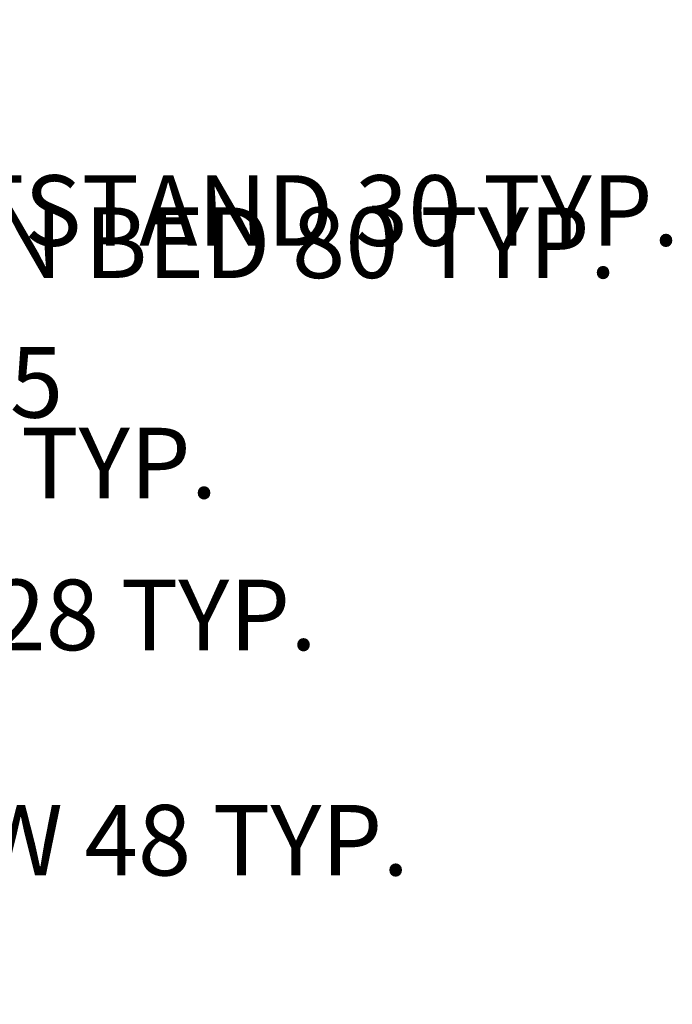
# Model space of a CAD drawing. Units: inches. Extents: x 1173 to 2157, y 515 to 1129.
# Tile 13 of 13: x 1824 to 2157, y 578 to 1080. Entities that reach past the tile are written whole.
import ezdxf

# ---------------------------------------------------------------- set-up
doc = ezdxf.new("R2010")
doc.units = ezdxf.units.IN
doc.header["$MEASUREMENT"] = 0
doc.layers.add('A-ANNO-DIMS', color=2, linetype='Continuous', lineweight=18)
doc.styles.get("Standard").update_dxf_attribs({"font": 'arial.ttf'})
doc.dimstyles.get("Standard").update_dxf_attribs({"dimtxt": 36, "dimasz": 0.18, "dimexe": 0.18, "dimexo": 0.0625, "dimgap": 0.09, "dimtad": 0, "dimtih": 1, "dimtoh": 1, "dimdec": 0, "dimrnd": 72, "dimzin": 0, "dimdsep": 46, "dimlunit": 3, "dimtxsty": 'Standard', "dimcen": 2, "dimadec": 0, "dimazin": 0, "dimtfac": 1, "dimtdec": 0, "dimtofl": 0, "dimtmove": 0, "dimatfit": 3, "dimfxl": 1, "dimtolj": 1, "dimtzin": 0, "dimarcsym": 0})

# ---------------------------------------------------------------- blocks, each defined once
blk = doc.blocks.new('*D26')
at = {"layer": 'A-ANNO-DIMS', "color": 0, "lineweight": -2, "transparency": 16777216}
for p, q in [((1577.15, 654.34), (1577.15, 661.66)), ((1577.33, 661.48), (1624.97, 661.48)), ((1625.15, 654.34), (1625.15, 661.66)), ((1625.15, 661.48), (1625.33, 661.48))]:
    blk.add_line(p, q, dxfattribs=at)
at = {"layer": 'A-ANNO-DIMS', "color": 0, "transparency": 16777216}
for points in [[(1577.33, 661.51), (1577.33, 661.45), (1577.15, 661.48)], [(1624.97, 661.51), (1624.97, 661.45), (1625.15, 661.48)]]:
    blk.add_solid(points, dxfattribs=at)
at = {"layer": 'Defpoints', "color": 0, "transparency": 16777216}
for p in [(1625.15, 661.48), (1577.15, 654.28), (1625.15, 654.28)]:
    blk.add_point(p, dxfattribs=at)
at = {"layer": 'A-ANNO-DIMS', "color": 0, "transparency": 16777216, "insert": (1831.09, 661.48), "char_height": 36, "attachment_point": 5}
blk.add_mtext('\\A1;WINDOW 48 TYP.', dxfattribs=at)
blk = doc.blocks.new('*D28')
at = {"layer": 'A-ANNO-DIMS', "color": 0, "lineweight": -2, "transparency": 16777216}
for p, q in [((1581.66, 978.31), (1581.66, 966.19)), ((1661.66, 978.31), (1661.66, 966.19)), ((1581.84, 966.37), (1661.48, 966.37)), ((1661.66, 966.37), (1661.84, 966.37))]:
    blk.add_line(p, q, dxfattribs=at)
at = {"layer": 'A-ANNO-DIMS', "color": 0, "transparency": 16777216}
for points in [[(1581.84, 966.4), (1581.84, 966.34), (1581.66, 966.37)], [(1661.48, 966.4), (1661.48, 966.34), (1661.66, 966.37)]]:
    blk.add_solid(points, dxfattribs=at)
at = {"layer": 'Defpoints', "color": 0, "transparency": 16777216}
for p in [(1581.66, 978.37), (1661.66, 978.37), (1661.66, 966.37)]:
    blk.add_point(p, dxfattribs=at)
at = {"layer": 'A-ANNO-DIMS', "color": 0, "transparency": 16777216, "insert": (1904.61, 966.37), "char_height": 36, "attachment_point": 5}
blk.add_mtext('\\A1;QUEEN BED 80 TYP.', dxfattribs=at)
blk = doc.blocks.new('*D32')
at = {"layer": 'A-ANNO-DIMS', "color": 0, "lineweight": -2, "transparency": 16777216}
for p, q in [((1632.82, 772.28), (1632.82, 776.62)), ((1633, 776.44), (1660.73, 776.44)), ((1660.91, 772.28), (1660.91, 776.62)), ((1660.91, 776.44), (1661.09, 776.44))]:
    blk.add_line(p, q, dxfattribs=at)
at = {"layer": 'A-ANNO-DIMS', "color": 0, "transparency": 16777216}
for points in [[(1633, 776.47), (1633, 776.41), (1632.82, 776.44)], [(1660.73, 776.47), (1660.73, 776.41), (1660.91, 776.44)]]:
    blk.add_solid(points, dxfattribs=at)
at = {"layer": 'Defpoints', "color": 0, "transparency": 16777216}
for p in [(1660.91, 776.44), (1632.82, 772.22), (1660.91, 772.22)]:
    blk.add_point(p, dxfattribs=at)
at = {"layer": 'A-ANNO-DIMS', "color": 0, "transparency": 16777216, "insert": (1823.46, 776.44), "char_height": 36, "attachment_point": 5}
blk.add_mtext('\\A1;LAMP 28 TYP.', dxfattribs=at)
blk = doc.blocks.new('*D34')
at = {"layer": 'A-ANNO-DIMS', "color": 0, "lineweight": -2, "transparency": 16777216}
for p, q in [((1631.9, 978.41), (1631.9, 982.97)), ((1632.08, 982.79), (1661.32, 982.79)), ((1661.5, 978.41), (1661.5, 982.97)), ((1661.5, 982.79), (1661.68, 982.79))]:
    blk.add_line(p, q, dxfattribs=at)
at = {"layer": 'A-ANNO-DIMS', "color": 0, "transparency": 16777216}
for points in [[(1632.08, 982.82), (1632.08, 982.76), (1631.9, 982.79)], [(1661.32, 982.82), (1661.32, 982.76), (1661.5, 982.79)]]:
    blk.add_solid(points, dxfattribs=at)
at = {"layer": 'Defpoints', "color": 0, "transparency": 16777216}
for p in [(1661.5, 982.79), (1631.9, 978.35), (1661.5, 978.35)]:
    blk.add_point(p, dxfattribs=at)
at = {"layer": 'A-ANNO-DIMS', "color": 0, "transparency": 16777216, "insert": (1918.96, 982.79), "char_height": 36, "attachment_point": 5}
blk.add_mtext('\\A1;NIGHTSTAND 30 TYP.', dxfattribs=at)
blk = doc.blocks.new('*D44')
at = {"layer": 'A-ANNO-DIMS', "color": 0, "lineweight": -2, "transparency": 16777216}
for p, q in [((1630.26, 849.3), (1630.26, 854.13)), ((1630.44, 853.95), (1661.48, 853.95)), ((1661.66, 849.3), (1661.66, 854.13)), ((1661.66, 853.95), (1661.84, 853.95))]:
    blk.add_line(p, q, dxfattribs=at)
at = {"layer": 'A-ANNO-DIMS', "color": 0, "transparency": 16777216}
for points in [[(1630.44, 853.98), (1630.44, 853.92), (1630.26, 853.95)], [(1661.48, 853.98), (1661.48, 853.92), (1661.66, 853.95)]]:
    blk.add_solid(points, dxfattribs=at)
at = {"layer": 'Defpoints', "color": 0, "transparency": 16777216}
for p in [(1630.26, 849.24), (1661.66, 853.95), (1661.66, 849.24)]:
    blk.add_point(p, dxfattribs=at)
at = {"layer": 'A-ANNO-DIMS', "color": 0, "transparency": 16777216, "insert": (1799.17, 853.95), "char_height": 36, "attachment_point": 5}
blk.add_mtext('\\A1;WC 31 TYP.', dxfattribs=at)
blk = doc.blocks.new('*D100')
at = {"layer": 'A-ANNO-DIMS', "color": 0, "lineweight": -2, "transparency": 16777216}
for p, q in [((1661.73, 894.92), (1696.15, 894.92)), ((1695.97, 894.92), (1695.97, 895.1)), ((1695.97, 895.1), (1696.15, 895.1)), ((1695.97, 864.46), (1695.97, 894.74)), ((1661.73, 864.28), (1696.15, 864.28))]:
    blk.add_line(p, q, dxfattribs=at)
at = {"layer": 'A-ANNO-DIMS', "color": 0, "transparency": 16777216}
for points in [[(1695.94, 894.74), (1696, 894.74), (1695.97, 894.92)], [(1695.94, 864.46), (1696, 864.46), (1695.97, 864.28)]]:
    blk.add_solid(points, dxfattribs=at)
at = {"layer": 'Defpoints', "color": 0, "transparency": 16777216}
for p in [(1661.66, 894.92), (1695.97, 894.92), (1661.66, 864.28)]:
    blk.add_point(p, dxfattribs=at)
at = {"layer": 'A-ANNO-DIMS', "color": 0, "transparency": 16777216, "insert": (1771.08, 895.1), "char_height": 36, "attachment_point": 5}
blk.add_mtext('\\A1;30.635', dxfattribs=at)

msp = doc.modelspace()

# ---------------------------------------------------------------- dimensions: what is measured, and where the dimension line sits
at = {"layer": 'A-ANNO-DIMS'}
for base, p1, p2, text, picture, middle in [((1661.6635, 966.3712), (1581.6634, 978.3712), (1661.6635, 978.3712), 'QUEEN BED <> TYP.', '*D28', (1904.6142, 966.3712)), ((1661.5047, 982.7919), (1631.9047, 978.3519), (1661.5047, 978.3519), 'NIGHTSTAND <> TYP.', '*D34', (1918.9562, 982.7919)), ((1661.6635, 853.9514), (1630.2601, 849.2409), (1661.6635, 849.2409), 'WC <> TYP.', '*D44', (1799.1681, 853.9514)), ((1660.9104, 776.4354), (1632.8165, 772.2213), (1660.9104, 772.2213), 'LAMP <> TYP.', '*D32', (1823.4628, 776.4354)), ((1625.1498, 661.4805), (1577.1498, 654.2805), (1625.1498, 654.2805), 'WINDOW <> TYP.', '*D26', (1831.0938, 661.4805))]:
    dim = msp.add_linear_dim(base=base, p1=p1, p2=p2, text=text, dimstyle='Standard', override={"dimdec": 0, "dimlfac": 1, "dimrnd": 0, "dimzin": 0, "dimdsep": 46, "dimlunit": 2}, dxfattribs=at)
    dim.commit()
    dim.dimension.update_dxf_attribs({"geometry": picture, "text_midpoint": middle})
dim = msp.add_linear_dim(base=(1695.966, 894.9156), p1=(1661.6635, 864.2805), p2=(1661.6635, 894.9156), angle=90, dimstyle='Standard', override={"dimdec": 3, "dimlfac": 1, "dimrnd": 0, "dimzin": 0, "dimdsep": 46, "dimlunit": 2}, dxfattribs=at)
dim.commit()
dim.dimension.update_dxf_attribs({"geometry": '*D100', "text_midpoint": (1771.0845, 895.0956)})

doc.saveas('drawing.dxf')
